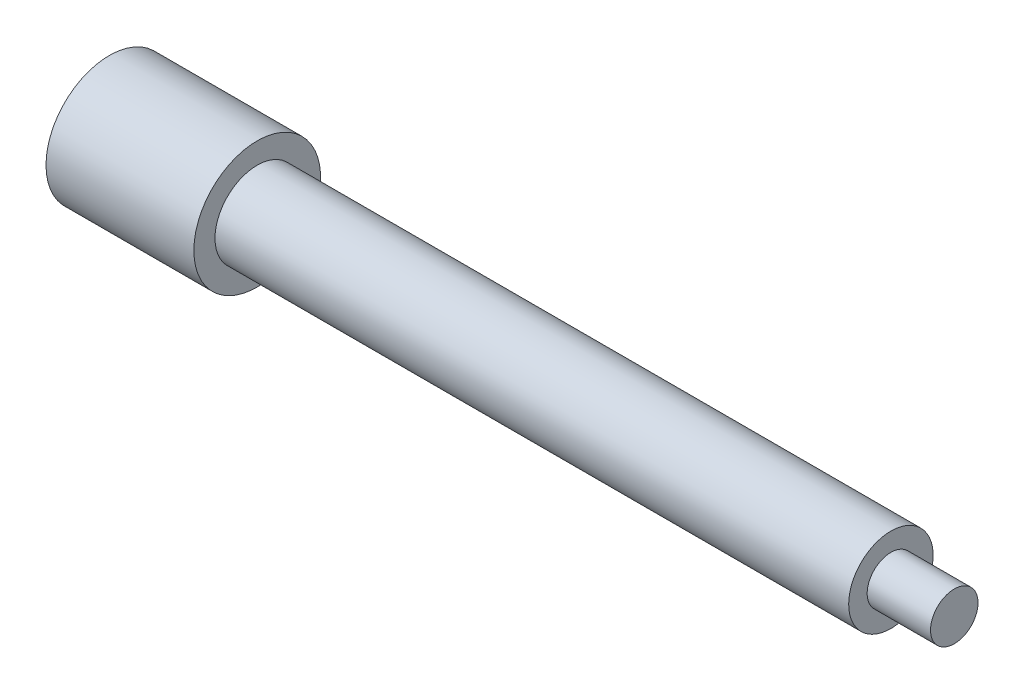
from build123d import *


with BuildPart() as part:
    # Stepped Shaft Profile → Stepped Shaft Revolve (revolve)
    with BuildSketch(Plane.XY, mode=Mode.PRIVATE) as stepped_shaft_revolve_sk:
        Polygon((0, 0), (0, 6), (14, 6), (14, 4), (74, 4), (74, 2.25), (80, 2.25), (80, 0), align=None)
    revolve(stepped_shaft_revolve_sk.sketch.rotate(Axis((0, 0, 0), (1, 0, 0)), 90), axis=Axis((0, 0, 0), (1, 0, 0)))


solid = part.part
